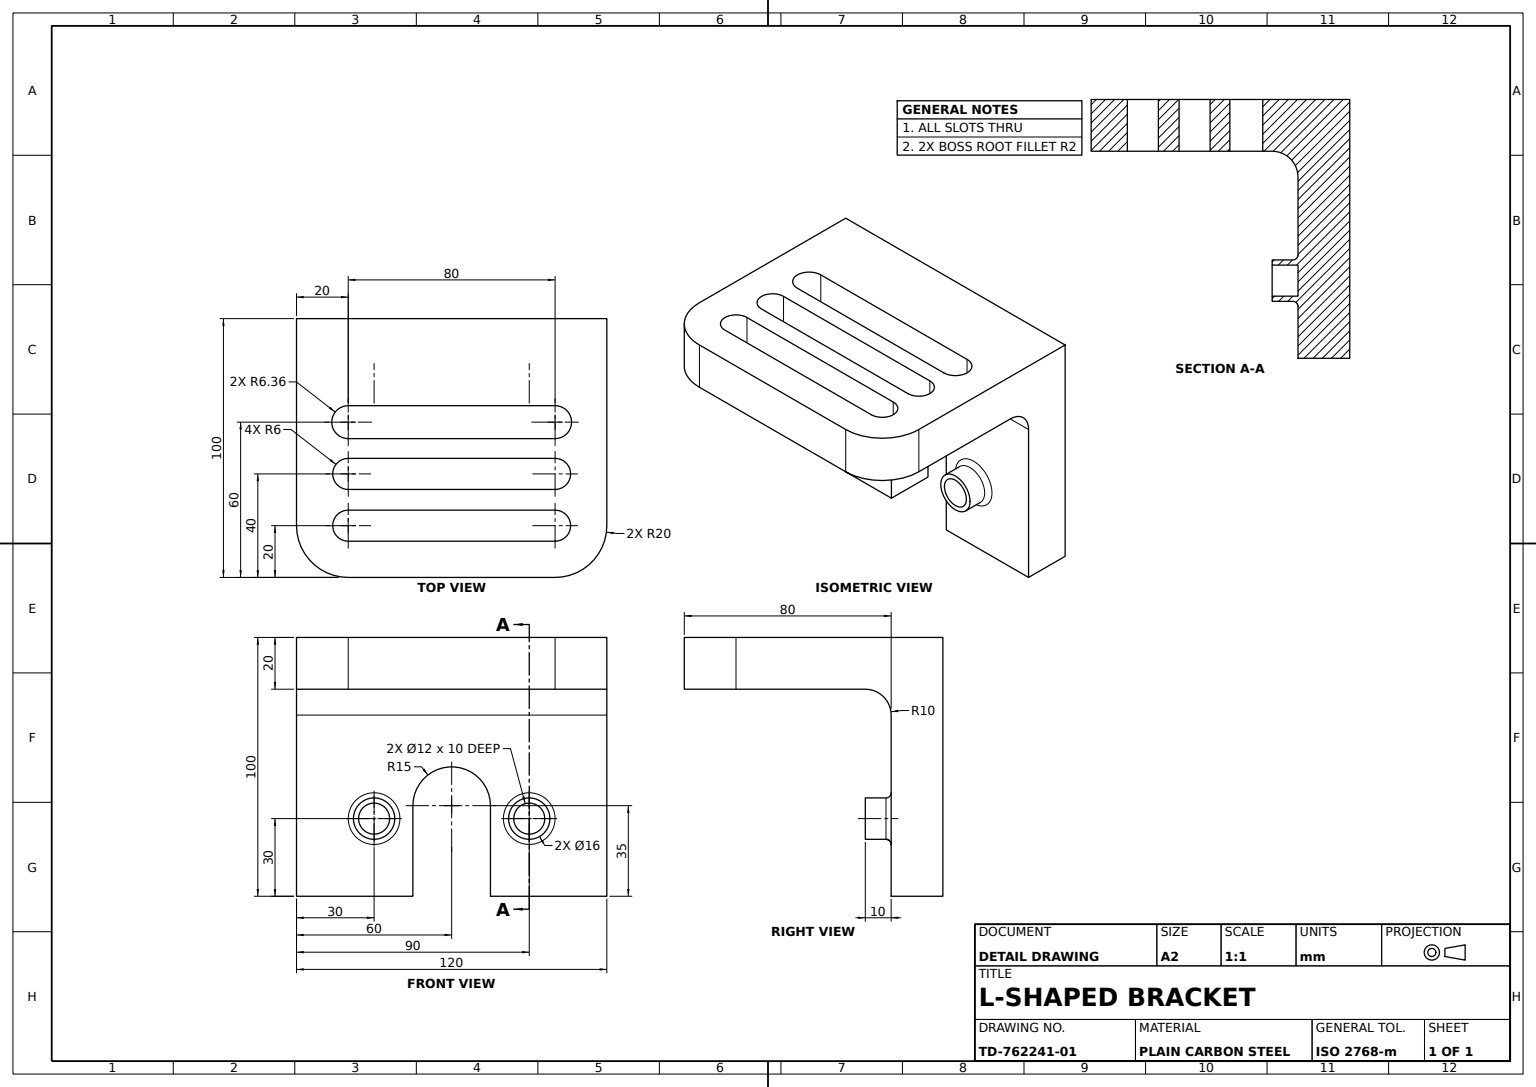
from build123d import *

# Parameters (mm, degrees)
BACK_PLATE_PROFILE_W        = 120
BACK_PLATE_PROFILE_H        = 100
BACK_PLATE_120X100X20_DEPTH = 20
TOP_ARM_PROFILE_W           = 120
TOP_ARM_PROFILE_H           = 20
TOP_ARM_80_DEPTH            = 80
SLOT_1_CUT_DEPTH            = 176.499287748
SLOT_2_CUT_DEPTH            = 176.499287748
SLOT_3_CUT_DEPTH            = 176.499287748
ARM_ROOT_FILLET_R10_R       = 10
ARM_CORNER_ROUND_R20_R      = 20
BACK_PLATE_CUT_30_DEPTH     = 176.499287748
BOSS_A_SKETCH_R             = 8
BOSS_A_SKETCH_R_2           = 6
MOUNTING_BOSS_A_DEPTH       = 10
BOSS_B_SKETCH_R             = 8
BOSS_B_SKETCH_R_2           = 6
MOUNTING_BOSS_B_DEPTH       = 10
BOSS_EDGE_FILLET_R2_R       = 2


with BuildPart() as part:
    # Back Plate Profile → Back Plate 120x100x20 (new body)
    with BuildSketch(Plane.XY):
        with Locations((60, 50)):
            Rectangle(BACK_PLATE_PROFILE_W, BACK_PLATE_PROFILE_H)
    extrude(amount=BACK_PLATE_120X100X20_DEPTH)

    # Top Arm Profile → Top Arm 80 (add)
    with BuildSketch(Plane.XY.offset(20)):
        with Locations((60, 90)):
            Rectangle(TOP_ARM_PROFILE_W, TOP_ARM_PROFILE_H)
    extrude(amount=TOP_ARM_80_DEPTH)

    # Slot 1 Sketch → Slot 1 Cut (cut, through all)
    with BuildSketch(Plane.XZ.offset(-80)):
        with BuildLine():
            Line((20, 86), (100, 86))
            ThreePointArc((100, 86), (106, 80), (100, 74))
            Line((100, 74), (20, 74))
            ThreePointArc((20, 74), (14, 80), (20, 86))
        make_face()
    extrude(amount=-SLOT_1_CUT_DEPTH, mode=Mode.SUBTRACT)

    # Slot 2 Sketch → Slot 2 Cut (cut, through all)
    with BuildSketch(Plane.XZ.offset(-80)):
        with BuildLine():
            Line((20, 66), (100, 66))
            ThreePointArc((100, 66), (106, 60), (100, 54))
            Line((100, 54), (20, 54))
            ThreePointArc((20, 54), (14, 60), (20, 66))
        make_face()
    extrude(amount=-SLOT_2_CUT_DEPTH, mode=Mode.SUBTRACT)

    # Slot 3 Sketch → Slot 3 Cut (cut, through all)
    with BuildSketch(Plane.XZ.offset(-80)):
        with BuildLine():
            Line((20, 46.364855501), (100, 46.364855501))
            ThreePointArc((100, 46.364855501), (106.364855501, 40), (100, 33.635144499))
            Line((100, 33.635144499), (20, 33.635144499))
            ThreePointArc((20, 33.635144499), (13.635144499, 40), (20, 46.364855501))
        make_face()
    extrude(amount=-SLOT_3_CUT_DEPTH, mode=Mode.SUBTRACT)

    # Arm Root Fillet R10
    arm_root_fillet_r10_edges = [part.edges().sort_by_distance(p)[0] for p in [
        (60, 80, 20),
    ]]
    fillet(arm_root_fillet_r10_edges, radius=ARM_ROOT_FILLET_R10_R)

    # Arm Corner Round R20
    arm_corner_round_r20_edges = [part.edges().sort_by_distance(p)[0] for p in [
        (0, 90, 100),
        (120, 90, 100),
    ]]
    fillet(arm_corner_round_r20_edges, radius=ARM_CORNER_ROUND_R20_R)

    # Back Plate Cut Sketch → Back Plate Cut 30 (cut, through all)
    with BuildSketch(Plane.XY.offset(20)):
        with BuildLine():
            Line((45, 35), (45, 0))
            Line((45, 0), (75, 0))
            Line((75, 0), (75, 35))
            ThreePointArc((75, 35), (60, 50), (45, 35))
        make_face()
    extrude(amount=-BACK_PLATE_CUT_30_DEPTH, mode=Mode.SUBTRACT)

    # Boss A Sketch → Mounting Boss A (add)
    with BuildSketch(Plane.XY.offset(20)):
        with Locations((30, 30)):
            Circle(BOSS_A_SKETCH_R)
        with Locations((30, 30)):
            Circle(BOSS_A_SKETCH_R_2, mode=Mode.SUBTRACT)
    extrude(amount=MOUNTING_BOSS_A_DEPTH)

    # Boss B Sketch → Mounting Boss B (add)
    with BuildSketch(Plane.XY.offset(20)):
        with Locations((90, 30)):
            Circle(BOSS_B_SKETCH_R)
        with Locations((90, 30)):
            Circle(BOSS_B_SKETCH_R_2, mode=Mode.SUBTRACT)
    extrude(amount=MOUNTING_BOSS_B_DEPTH)

    # Boss Edge Fillet R2
    boss_edge_fillet_r2_edges = [part.edges().sort_by_distance(p)[0] for p in [
        (22, 30, 20),
        (82, 30, 20),
    ]]
    fillet(boss_edge_fillet_r2_edges, radius=BOSS_EDGE_FILLET_R2_R)


solid = part.part
